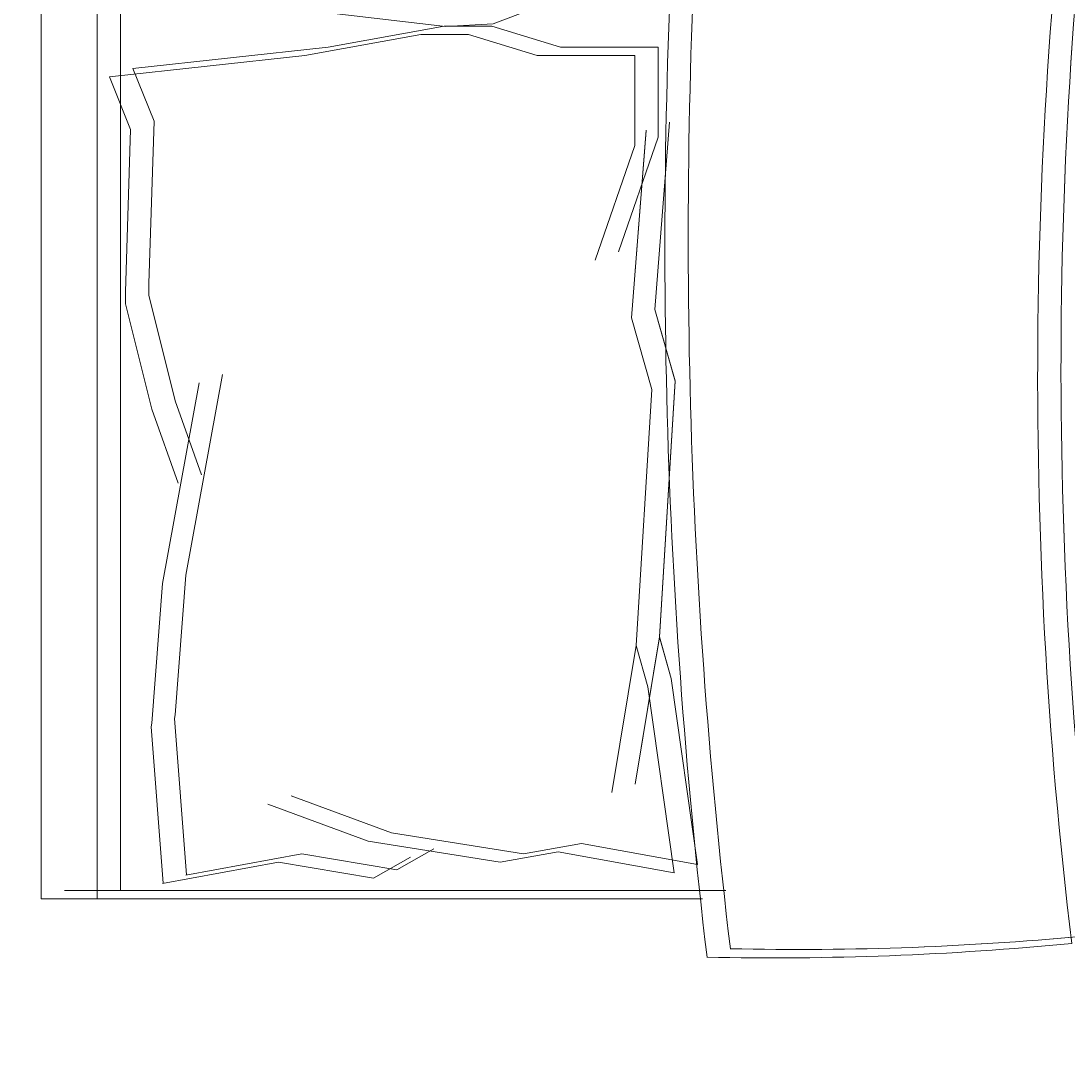
# Model space of a CAD drawing. Units: inches. Extents: x 1962 to 2771, y 1245 to 2660.
# Tile 43 of 114: x 2093.47 to 2116.25, y 2075.47 to 2098.32. Entities that reach past the tile are written whole.
import ezdxf

# ---------------------------------------------------------------- set-up
doc = ezdxf.new("R2010")
doc.units = ezdxf.units.IN
doc.layers.add('A-ANNO-DIMS', color=2, linetype='Continuous', lineweight=18)
doc.layers.add('A-FURN', color=8, linetype='Continuous', lineweight=13)
doc.styles.get("Standard").update_dxf_attribs({"font": 'arial.ttf'})
doc.dimstyles.get("Standard").update_dxf_attribs({"dimtxt": 0.18, "dimasz": 0.18, "dimexe": 0.18, "dimexo": 0.0625, "dimgap": 0.09, "dimtad": 0, "dimtih": 1, "dimtoh": 1, "dimdec": 4, "dimzin": 0, "dimdsep": 46, "dimtxsty": 'Standard', "dimcen": 0.09, "dimadec": 0, "dimazin": 0, "dimtfac": 1, "dimtdec": 4, "dimtofl": 0, "dimtmove": 0, "dimatfit": 3, "dimfxl": 1, "dimtolj": 1, "dimtzin": 0, "dimarcsym": 0})

# ---------------------------------------------------------------- blocks, each defined once
blk = doc.blocks.new('BED-PLAN')
for p, q in [((1.727, 2.945), (1.727, 40.933)), ((1.727, 2.945), (1.727, 40.933)), ((0, 2.764), (0, 40.751)), ((1.219, 2.764), (1.219, 40.752)), ((1.219, 2.763), (1.219, 40.751)), ((9.838, 21.81), (11.301, 22.362)), ((9.838, 21.81), (11.301, 22.362)), ((6.254, 22.046), (8.806, 21.745)), ((6.254, 22.046), (8.806, 21.745)), ((6.247, 21.296), (8.776, 21.755)), ((6.247, 21.296), (8.776, 21.755)), ((8.776, 21.755), (9.81, 21.755)), ((8.776, 21.755), (9.81, 21.755)), ((8.806, 21.745), (9.838, 21.81)), ((8.806, 21.745), (9.838, 21.81)), ((9.81, 21.755), (11.304, 21.296)), ((9.81, 21.755), (11.304, 21.296)), ((5.739, 21.114), (8.268, 21.574)), ((5.739, 21.114), (8.268, 21.574)), ((8.268, 21.574), (9.302, 21.574)), ((8.268, 21.574), (9.302, 21.574)), ((9.302, 21.574), (10.796, 21.114)), ((9.302, 21.574), (10.796, 21.114)), ((1.995, 20.836), (6.247, 21.296)), ((1.995, 20.836), (6.247, 21.296)), ((11.304, 21.296), (13.436, 21.296)), ((11.304, 21.296), (13.436, 21.296)), ((13.436, 21.296), (13.436, 19.342)), ((13.436, 21.296), (13.436, 19.342)), ((1.487, 20.655), (5.739, 21.114)), ((1.487, 20.654), (5.739, 21.114)), ((10.796, 21.114), (12.927, 21.114)), ((10.796, 21.114), (12.927, 21.114)), ((12.927, 21.114), (12.927, 19.161)), ((12.927, 21.114), (12.927, 19.161)), ((2.455, 19.687), (1.995, 20.836)), ((2.455, 19.687), (1.995, 20.836)), ((1.946, 19.506), (1.487, 20.655)), ((1.946, 19.505), (1.487, 20.654)), ((2.34, 16.153), (2.455, 19.687)), ((2.34, 16.153), (2.455, 19.687)), ((13.361, 15.591), (13.682, 19.67)), ((13.361, 15.591), (13.682, 19.67)), ((1.831, 15.972), (1.946, 19.506)), ((1.831, 15.972), (1.946, 19.505)), ((12.853, 15.409), (13.173, 19.489)), ((12.853, 15.409), (13.173, 19.488)), ((13.436, 19.342), (12.568, 16.843)), ((13.436, 19.342), (12.568, 16.843)), ((12.927, 19.161), (12.06, 16.661)), ((12.927, 19.161), (12.06, 16.661)), ((2.34, 15.898), (2.34, 16.153)), ((2.34, 15.897), (2.34, 16.153)), ((1.831, 15.716), (1.831, 15.972)), ((1.831, 15.716), (1.831, 15.972)), ((2.914, 13.6), (2.34, 15.898)), ((2.914, 13.599), (2.34, 15.897)), ((2.406, 13.418), (1.831, 15.716)), ((2.406, 13.418), (1.831, 15.716)), ((13.804, 14.033), (13.361, 15.591)), ((13.804, 14.032), (13.361, 15.591)), ((13.296, 13.851), (12.853, 15.409)), ((13.296, 13.851), (12.853, 15.409)), ((3.144, 9.808), (3.949, 14.174)), ((3.144, 9.807), (3.949, 14.174)), ((2.636, 9.626), (3.44, 13.993)), ((2.636, 9.626), (3.44, 13.992)), ((13.461, 8.461), (13.804, 14.033)), ((13.461, 8.46), (13.804, 14.032)), ((12.953, 8.279), (13.296, 13.851)), ((12.953, 8.279), (13.296, 13.851)), ((3.489, 11.991), (2.914, 13.6)), ((3.489, 11.991), (2.914, 13.599)), ((2.981, 11.809), (2.406, 13.418)), ((2.981, 11.809), (2.406, 13.418)), ((2.406, 6.587), (2.636, 9.626)), ((2.406, 6.587), (2.636, 9.626)), ((2.914, 6.768), (3.144, 9.808)), ((2.914, 6.768), (3.144, 9.807)), ((12.931, 5.256), (13.461, 8.461)), ((12.931, 5.255), (13.461, 8.46)), ((13.461, 8.461), (13.718, 7.56)), ((13.461, 8.46), (13.718, 7.56)), ((12.423, 5.074), (12.953, 8.279)), ((12.423, 5.074), (12.953, 8.279)), ((12.953, 8.279), (13.21, 7.378)), ((12.953, 8.279), (13.21, 7.378)), ((13.718, 7.56), (14.292, 3.509)), ((13.718, 7.56), (14.292, 3.508)), ((13.21, 7.378), (13.784, 3.327)), ((13.21, 7.378), (13.784, 3.327)), ((2.9, 6.685), (2.914, 6.768)), ((2.9, 6.684), (2.914, 6.768)), ((3.162, 3.282), (2.9, 6.685)), ((3.162, 3.282), (2.9, 6.684)), ((2.392, 6.503), (2.406, 6.587)), ((2.392, 6.503), (2.406, 6.587)), ((2.653, 3.1), (2.392, 6.503)), ((2.653, 3.1), (2.392, 6.503)), ((7.118, 4.016), (4.935, 4.821)), ((7.118, 4.016), (4.935, 4.821)), ((7.626, 4.198), (5.443, 5.002)), ((7.626, 4.198), (5.443, 5.002)), ((10.5, 3.738), (7.626, 4.198)), ((10.5, 3.738), (7.626, 4.198)), ((9.991, 3.557), (7.118, 4.016)), ((9.992, 3.557), (7.118, 4.016)), ((11.764, 3.968), (10.5, 3.738)), ((11.764, 3.968), (10.5, 3.738)), ((14.292, 3.509), (11.764, 3.968)), ((14.292, 3.508), (11.764, 3.968)), ((3.144, 3.279), (5.673, 3.738)), ((3.144, 3.279), (5.673, 3.738)), ((5.673, 3.738), (7.741, 3.394)), ((5.673, 3.738), (7.741, 3.393)), ((7.233, 3.212), (8.038, 3.672)), ((7.233, 3.212), (8.038, 3.672)), ((7.741, 3.394), (8.546, 3.853)), ((7.741, 3.393), (8.546, 3.853)), ((11.256, 3.787), (9.991, 3.557)), ((11.256, 3.786), (9.992, 3.557)), ((13.784, 3.327), (11.256, 3.787)), ((13.784, 3.327), (11.256, 3.786)), ((2.636, 3.097), (5.164, 3.557)), ((2.636, 3.097), (5.164, 3.557)), ((5.164, 3.557), (7.233, 3.212)), ((5.164, 3.557), (7.233, 3.212)), ((14.396, 2.764), (0, 2.764)), ((14.396, 2.763), (0, 2.763)), ((14.904, 2.945), (0.508, 2.945)), ((14.904, 2.945), (0.508, 2.945))]:
    blk.add_line(p, q)
for centre, radius, start, end in [((124.762, 14.297), 102.556, 171.78449, 186.90062), ((124.762, 14.296), 102.556, 171.78449, 186.90062), ((124.254, 14.115), 102.556, 171.78449, 186.90062), ((124.254, 14.115), 102.556, 171.78449, 186.90062), ((145.219, 17.161), 131.131, 176.08655, 186.78213), ((145.219, 17.161), 131.131, 176.08655, 186.78213), ((144.711, 16.979), 131.131, 176.08655, 186.78213), ((144.711, 16.979), 131.131, 176.08655, 186.78213), ((16.482, 67.877), 66.218, 268.72178, 275.60397), ((16.483, 67.877), 66.218, 268.72178, 275.60397), ((15.974, 67.695), 66.218, 268.72178, 275.60397), ((15.974, 67.695), 66.218, 268.72178, 275.60397)]:
    blk.add_arc(centre, radius, start, end)
blk = doc.blocks.new('*D40')
at = {"layer": 'A-ANNO-DIMS', "color": 0, "lineweight": -2, "transparency": 16777216}
for p, q in [((2072.02, 2033.906), (2072.02, 2583.474)), ((2660.807, 2524.406), (2660.807, 2583.474)), ((2072.2, 2583.294), (2366.02, 2583.294)), ((2660.627, 2583.294), (2366.808, 2583.294))]:
    blk.add_line(p, q, dxfattribs=at)
at = {"layer": 'A-ANNO-DIMS', "color": 0, "transparency": 16777216}
for points in [[(2072.2, 2583.324), (2072.2, 2583.264), (2072.02, 2583.294)], [(2660.627, 2583.324), (2660.627, 2583.264), (2660.807, 2583.294)]]:
    blk.add_solid(points, dxfattribs=at)
at = {"layer": 'Defpoints', "color": 0, "transparency": 16777216}
for p in [(2660.807, 2583.294), (2660.807, 2524.344), (2072.02, 2033.844)]:
    blk.add_point(p, dxfattribs=at)
at = {"layer": 'A-ANNO-DIMS', "color": 0, "transparency": 16777216, "insert": (2366.414, 2583.294), "char_height": 0.18, "attachment_point": 5}
blk.add_mtext('\\A1;588.8', dxfattribs=at)

msp = doc.modelspace()

# ---------------------------------------------------------------- block references
at = {"layer": 'A-FURN'}
msp.add_blockref('BED-PLAN', (2093.917, 2076.454), dxfattribs=at)

# ---------------------------------------------------------------- dimensions: what is measured, and where the dimension line sits
at = {"layer": 'A-ANNO-DIMS'}
dim = msp.add_linear_dim(base=(2660.8074, 2583.2937), p1=(2072.0204, 2033.8437), p2=(2660.8074, 2524.3437), dimstyle='Standard', override={"dimdec": 1, "dimlfac": 1, "dimrnd": 0, "dimzin": 0, "dimdsep": 46, "dimlunit": 2}, dxfattribs=at)
dim.commit()
dim.dimension.update_dxf_attribs({"geometry": '*D40', "text_midpoint": (2366.4139, 2583.2937)})

doc.saveas('drawing.dxf')
